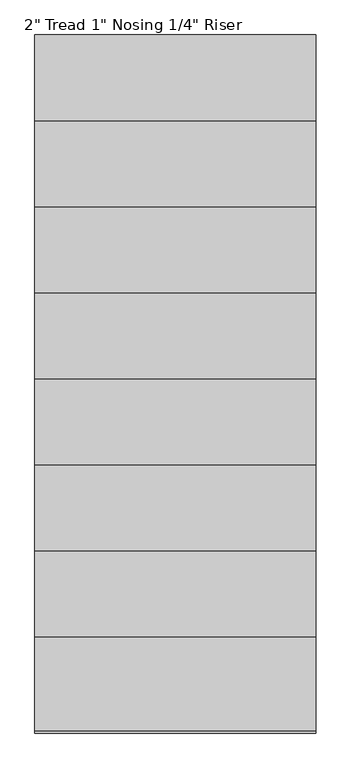
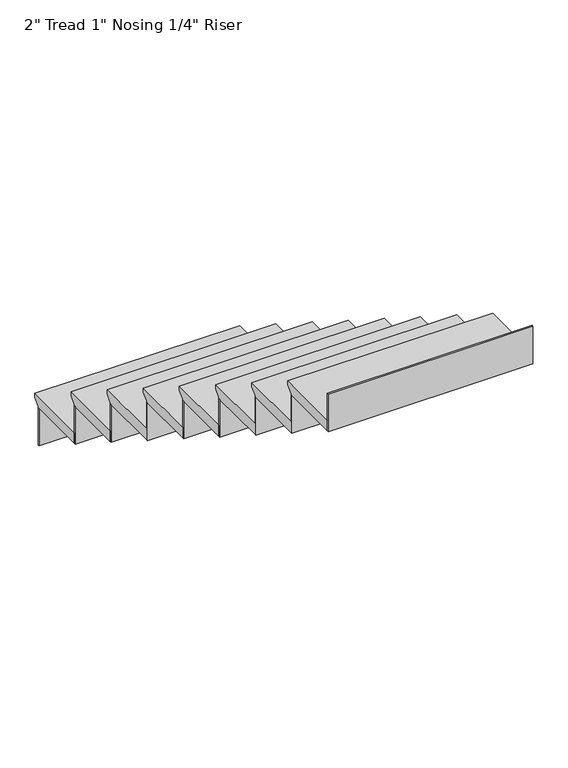
"""IFC4 building model written with IfcOpenShell, lengths in millimetres: stair flight geometry."""

from ifc_helpers import new_model, si_unit, frame, origin, place, context, project, spatial, polyline, outline, extrude, source, transform, mapped, element, save


def stair_flight_b9007331(model_context):
    return source(origin(), model_context, "Body", "SweptSolid", [
        extrude(outline(polyline([(8107.643496, 2387.6), (8412.443496, 2387.6), (8412.443496, 2368.55), (8387.043496, 2343.15), (8387.043496, 2336.8), (8107.643496, 2336.8), (8107.643496, 2387.6)])), frame((-11538.468339, 0.0, 0.0), z_axis=(1.0, 0.0, 0.0), x_axis=(0.0, 1.0, 0.0)), (0.0, 0.0, 1.0), 914.4),
        extrude(outline(polyline([(-11538.468339, 8380.693496), (-11538.468339, 8387.043496), (-10624.068339, 8387.043496), (-10624.068339, 8380.693496), (-11538.468339, 8380.693496)])), frame((0.0, 0.0, 2159.0), z_axis=(0.0, 0.0, 1.0), x_axis=(1.0, 0.0, 0.0)), (0.0, 0.0, 1.0), 177.8),
        extrude(outline(polyline([(-11538.468339, 8101.293496), (-11538.468339, 8107.643496), (-10624.068339, 8107.643496), (-10624.068339, 8101.293496), (-11538.468339, 8101.293496)])), frame((0.0, 0.0, 2336.8), z_axis=(0.0, 0.0, 1.0), x_axis=(1.0, 0.0, 0.0)), (0.0, 0.0, 1.0), 177.8),
        extrude(outline(polyline([(7828.243496, 2565.4), (8133.043496, 2565.4), (8133.043496, 2546.35), (8107.643496, 2520.95), (8107.643496, 2514.6), (7828.243496, 2514.6), (7828.243496, 2565.4)])), frame((-11538.468339, 0.0, 0.0), z_axis=(1.0, 0.0, 0.0), x_axis=(0.0, 1.0, 0.0)), (0.0, 0.0, 1.0), 914.4),
        extrude(outline(polyline([(-11538.468339, 7821.893496), (-11538.468339, 7828.243496), (-10624.068339, 7828.243496), (-10624.068339, 7821.893496), (-11538.468339, 7821.893496)])), frame((0.0, 0.0, 2514.6), z_axis=(0.0, 0.0, 1.0), x_axis=(1.0, 0.0, 0.0)), (0.0, 0.0, 1.0), 177.8),
        extrude(outline(polyline([(7548.843496, 2743.2), (7853.643496, 2743.2), (7853.643496, 2724.15), (7828.243496, 2698.75), (7828.243496, 2692.4), (7548.843496, 2692.4), (7548.843496, 2743.2)])), frame((-11538.468339, 0.0, 0.0), z_axis=(1.0, 0.0, 0.0), x_axis=(0.0, 1.0, 0.0)), (0.0, 0.0, 1.0), 914.4),
        extrude(outline(polyline([(-11538.468339, 7542.493496), (-11538.468339, 7548.843496), (-10624.068339, 7548.843496), (-10624.068339, 7542.493496), (-11538.468339, 7542.493496)])), frame((0.0, 0.0, 2692.4), z_axis=(0.0, 0.0, 1.0), x_axis=(1.0, 0.0, 0.0)), (0.0, 0.0, 1.0), 177.8),
        extrude(outline(polyline([(7269.443496, 2921.0), (7574.243496, 2921.0), (7574.243496, 2901.95), (7548.843496, 2876.55), (7548.843496, 2870.2), (7269.443496, 2870.2), (7269.443496, 2921.0)])), frame((-11538.468339, 0.0, 0.0), z_axis=(1.0, 0.0, 0.0), x_axis=(0.0, 1.0, 0.0)), (0.0, 0.0, 1.0), 914.4),
        extrude(outline(polyline([(-11538.468339, 7263.093496), (-11538.468339, 7269.443496), (-10624.068339, 7269.443496), (-10624.068339, 7263.093496), (-11538.468339, 7263.093496)])), frame((0.0, 0.0, 2870.2), z_axis=(0.0, 0.0, 1.0), x_axis=(1.0, 0.0, 0.0)), (0.0, 0.0, 1.0), 177.8),
        extrude(outline(polyline([(6990.043496, 3098.8), (7294.843496, 3098.8), (7294.843496, 3079.75), (7269.443496, 3054.35), (7269.443496, 3048.0), (6990.043496, 3048.0), (6990.043496, 3098.8)])), frame((-11538.468339, 0.0, 0.0), z_axis=(1.0, 0.0, 0.0), x_axis=(0.0, 1.0, 0.0)), (0.0, 0.0, 1.0), 914.4),
        extrude(outline(polyline([(-11538.468339, 6983.693496), (-11538.468339, 6990.043496), (-10624.068339, 6990.043496), (-10624.068339, 6983.693496), (-11538.468339, 6983.693496)])), frame((0.0, 0.0, 3048.0), z_axis=(0.0, 0.0, 1.0), x_axis=(1.0, 0.0, 0.0)), (0.0, 0.0, 1.0), 177.8),
        extrude(outline(polyline([(6710.643496, 3276.6), (7015.443496, 3276.6), (7015.443496, 3257.55), (6990.043496, 3232.15), (6990.043496, 3225.8), (6710.643496, 3225.8), (6710.643496, 3276.6)])), frame((-11538.468339, 0.0, 0.0), z_axis=(1.0, 0.0, 0.0), x_axis=(0.0, 1.0, 0.0)), (0.0, 0.0, 1.0), 914.4),
        extrude(outline(polyline([(-11538.468339, 6704.293496), (-11538.468339, 6710.643496), (-10624.068339, 6710.643496), (-10624.068339, 6704.293496), (-11538.468339, 6704.293496)])), frame((0.0, 0.0, 3225.8), z_axis=(0.0, 0.0, 1.0), x_axis=(1.0, 0.0, 0.0)), (0.0, 0.0, 1.0), 177.8),
        extrude(outline(polyline([(6431.243496, 3454.4), (6736.043496, 3454.4), (6736.043496, 3435.35), (6710.643496, 3409.95), (6710.643496, 3403.6), (6431.243496, 3403.6), (6431.243496, 3454.4)])), frame((-11538.468339, 0.0, 0.0), z_axis=(1.0, 0.0, 0.0), x_axis=(0.0, 1.0, 0.0)), (0.0, 0.0, 1.0), 914.4),
        extrude(outline(polyline([(-11538.468339, 6424.893496), (-11538.468339, 6431.243496), (-10624.068339, 6431.243496), (-10624.068339, 6424.893496), (-11538.468339, 6424.893496)])), frame((0.0, 0.0, 3403.6), z_axis=(0.0, 0.0, 1.0), x_axis=(1.0, 0.0, 0.0)), (0.0, 0.0, 1.0), 177.8),
        extrude(outline(polyline([(-11538.468339, 6145.493496), (-11538.468339, 6151.843496), (-10624.068339, 6151.843496), (-10624.068339, 6145.493496), (-11538.468339, 6145.493496)])), frame((0.0, 0.0, 3581.4), z_axis=(0.0, 0.0, 1.0), x_axis=(1.0, 0.0, 0.0)), (0.0, 0.0, 1.0), 177.8),
        extrude(outline(polyline([(6151.843496, 3632.2), (6456.643496, 3632.2), (6456.643496, 3613.15), (6431.243496, 3587.75), (6431.243496, 3581.4), (6151.843496, 3581.4), (6151.843496, 3632.2)])), frame((-11538.468339, 0.0, 0.0), z_axis=(1.0, 0.0, 0.0), x_axis=(0.0, 1.0, 0.0)), (0.0, 0.0, 1.0), 914.4),
    ])


if __name__ == "__main__":
    model = new_model("IFC4")
    model_context = context("Model", 3, world=origin())
    ifc_project = project(units=[si_unit("LENGTHUNIT", "METRE", prefix="MILLI")], contexts=[model_context])
    site = spatial("IfcSite", under=ifc_project)
    building = spatial("IfcBuilding", under=site)
    placement = place(None, origin())
    stair_flight_shape = stair_flight_b9007331(model_context)
    element("IfcStairFlight", 1, ObjectType="2\" Tread 1\" Nosing 1/4\" Riser", at=placement, inside=building, context=model_context, shape_type="MappedRepresentation", body=[
        mapped(stair_flight_shape, transform((0.0, 0.0, 0.0), x_axis=(1.0, 0.0, 0.0), y_axis=(0.0, 1.0, 0.0), z_axis=(0.0, 0.0, 1.0))),
    ])
    save(model, "model.ifc")
